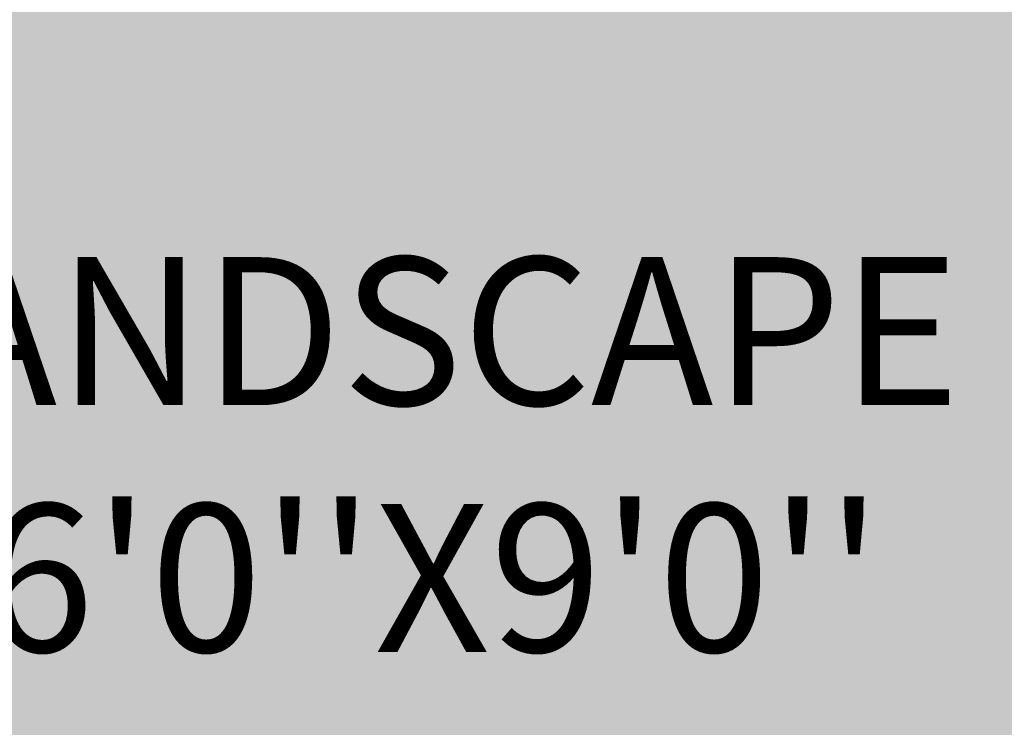
# Model space of a CAD drawing. Units: inches. Extents: x 84 to 1044, y -280 to 906.
# Tile 94 of 105: x 779 to 826, y 445 to 479. Entities that reach past the tile are written whole.
import ezdxf

# ---------------------------------------------------------------- set-up
doc = ezdxf.new("R2010")
doc.units = ezdxf.units.IN
doc.layers.add('A-ANNO-DIMS', color=2, linetype='Continuous', lineweight=18)
doc.layers.add('A-AREA-IDEN', color=7, linetype='Continuous', lineweight=13)
doc.layers.add('L-PLNT-PATT', color=9, linetype='Continuous', lineweight=9, true_color=0xafd9aa)
doc.styles.add('1-100DIM', font='txt', dxfattribs={"height": 0.3})
doc.styles.get("Standard").update_dxf_attribs({"font": 'arial.ttf'})
doc.dimstyles.get("Standard").update_dxf_attribs({"dimtxt": 0.18, "dimasz": 0.18, "dimexe": 0.18, "dimexo": 0.0625, "dimgap": 0.09, "dimtad": 0, "dimtih": 1, "dimtoh": 1, "dimdec": 4, "dimzin": 0, "dimdsep": 46, "dimtxsty": 'Standard', "dimcen": 0.09, "dimadec": 0, "dimazin": 0, "dimtfac": 1, "dimtdec": 4, "dimtofl": 0, "dimtmove": 0, "dimatfit": 3, "dimfxl": 1, "dimtolj": 1, "dimtzin": 0, "dimarcsym": 0})

# ---------------------------------------------------------------- blocks, each defined once
blk = doc.blocks.new('*D62')
at = {"layer": 'A-ANNO-DIMS', "color": 0, "lineweight": -2, "transparency": 16777216}
for p, q in [((203.179, 709.183), (203.179, 905.9)), ((203.359, 905.72), (549.232, 905.72)), ((895.894, 905.72), (550.021, 905.72)), ((896.074, 400.183), (896.074, 905.9))]:
    blk.add_line(p, q, dxfattribs=at)
at = {"layer": 'A-ANNO-DIMS', "color": 0, "transparency": 16777216}
for points in [[(203.359, 905.75), (203.359, 905.69), (203.179, 905.72)], [(895.894, 905.75), (895.894, 905.69), (896.074, 905.72)]]:
    blk.add_solid(points, dxfattribs=at)
at = {"layer": 'Defpoints', "color": 0, "transparency": 16777216}
for p in [(896.074, 905.72), (203.179, 709.12), (896.074, 400.12)]:
    blk.add_point(p, dxfattribs=at)
at = {"layer": 'A-ANNO-DIMS', "color": 0, "transparency": 16777216, "insert": (549.627, 905.72), "char_height": 0.18, "attachment_point": 5}
blk.add_mtext('\\A1;692.9', dxfattribs=at)

msp = doc.modelspace()

# ---------------------------------------------------------------- hatches: boundary and pattern name
at = {"layer": 'L-PLNT-PATT', "transparency": 33554597}
h = msp.add_hatch(color=256, dxfattribs=at)
h.dxf.hatch_style = 1
h.paths.add_polyline_path([(896.074, 511.12), (704.074, 511.12), (704.074, 491.62), (704.074, 419.62), (704.074, 400.12), (833.074, 400.12), (896.074, 400.12)])

# ---------------------------------------------------------------- texts
at = {"layer": 'A-AREA-IDEN', "insert": (769.898, 467.716), "char_height": 7, "attachment_point": 1, "style": '1-100DIM'}
msp.add_mtext_dynamic_manual_height_columns("{\\f@Malgun Gothic|b0|i0|c0|p34;LANDSCAPE\\P 16'0''X9'0''}", width=58.97918, gutter_width=15.851, heights=[0], dxfattribs=at)

# ---------------------------------------------------------------- dimensions: what is measured, and where the dimension line sits
at = {"layer": 'A-ANNO-DIMS'}
dim = msp.add_linear_dim(base=(896.074, 905.72), p1=(203.179, 709.12), p2=(896.074, 400.12), dimstyle='Standard', override={"dimdec": 1, "dimlfac": 1, "dimrnd": 0, "dimzin": 0, "dimdsep": 46, "dimlunit": 2}, dxfattribs=at)
dim.commit()
dim.dimension.update_dxf_attribs({"geometry": '*D62', "text_midpoint": (549.627, 905.72)})

doc.saveas('drawing.dxf')
